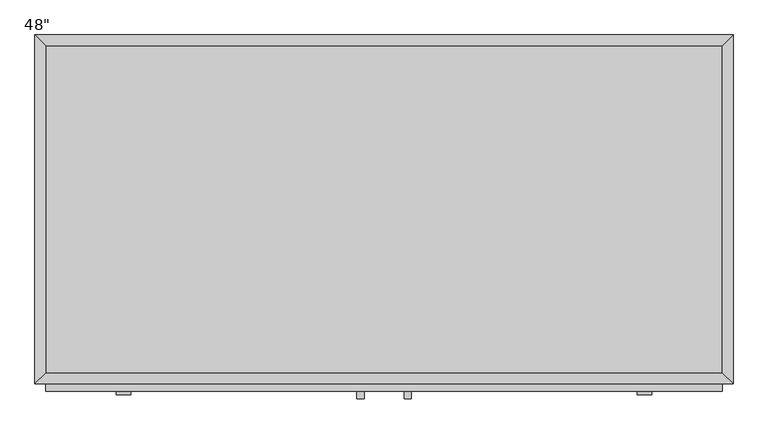
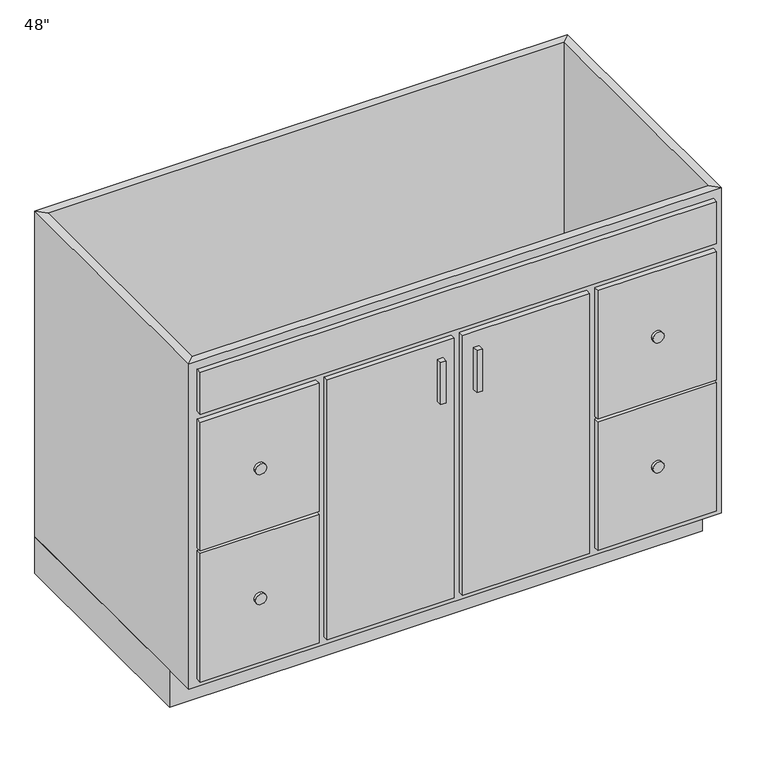
"""IFC4 building model written with IfcOpenShell, lengths in millimetres: furniture geometry."""

from ifc_helpers import new_model, si_unit, point, frame, frame_2d, origin, origin_with_axes, place, context, project, spatial, polyline, circle_curve, trimmed, segment, composite_curve, outline, extrude, faceted_brep, source, transform, mapped, element, save


def furniture_3428e43d(model_context):
    return source(origin(), model_context, "Body", "SolidModel", [
        extrude(outline(polyline([(700.44496, 0.0), (700.44496, -533.4), (-518.75504, -533.4), (-518.75504, 0.0), (700.44496, 0.0)])), origin_with_axes(), (0.0, 0.0, 1.0), 88.9),
        faceted_brep([(681.39496, -590.55, 876.3), (681.39496, -590.55, 88.9), (-499.70504, -590.55, 88.9), (-499.70504, -590.55, 876.3), (700.44496, -609.6, 876.3), (-518.75504, -609.6, 876.3), (700.44496, -609.6, 88.9), (-518.75504, -609.6, 88.9), (-499.70504, -19.05, 88.9), (-499.70504, -19.05, 876.3), (-518.75504, 0.0, 876.3), (-518.75504, 0.0, 88.9), (681.39496, -19.05, 88.9), (681.39496, -19.05, 876.3), (700.44496, 0.0, 876.3), (700.44496, 0.0, 88.9)], [[[0, 1, 2, 3]], [[4, 0, 3, 5]], [[6, 4, 5, 7]], [[1, 6, 7, 2]], [[3, 2, 8, 9]], [[5, 3, 9, 10]], [[7, 5, 10, 11]], [[2, 7, 11, 8]], [[9, 8, 12, 13]], [[10, 9, 13, 14]], [[11, 10, 14, 15]], [[8, 11, 15, 12]], [[13, 12, 1, 0]], [[14, 13, 0, 4]], [[15, 14, 4, 6]], [[12, 15, 6, 1]]]),
        extrude(outline(polyline([(681.39496, -19.05), (681.39496, -590.55), (-499.70504, -590.55), (-499.70504, -19.05), (681.39496, -19.05)])), frame((0.0, 0.0, 88.9), z_axis=(0.0, 0.0, 1.0), x_axis=(1.0, 0.0, 0.0)), (0.0, 0.0, 1.0), 19.05),
        extrude(outline(composite_curve([segment(trimmed(circle_curve(frame_2d((265.1125, 545.66371)), 12.7), [point((265.1125, 532.96371))], [point((265.1125, 558.36371))], False, "CARTESIAN"), True, "CONTINUOUS"), segment(trimmed(circle_curve(frame_2d((265.1125, 545.66371)), 12.7), [point((265.1125, 558.36371))], [point((265.1125, 532.96371))], False, "CARTESIAN"), True, "CONTINUOUS")], self_intersect=False)), frame((0.0, -628.65, 0.0), z_axis=(0.0, 1.0, 0.0), x_axis=(0.0, 0.0, 1.0)), (0.0, 0.0, 1.0), 6.35),
        extrude(outline(composite_curve([segment(trimmed(circle_curve(frame_2d((579.4375, 545.66371)), 12.7), [point((579.4375, 532.96371))], [point((579.4375, 558.36371))], False, "CARTESIAN"), True, "CONTINUOUS"), segment(trimmed(circle_curve(frame_2d((579.4375, 545.66371)), 12.7), [point((579.4375, 558.36371))], [point((579.4375, 532.96371))], False, "CARTESIAN"), True, "CONTINUOUS")], self_intersect=False)), frame((0.0, -628.65, 0.0), z_axis=(0.0, 1.0, 0.0), x_axis=(0.0, 0.0, 1.0)), (0.0, 0.0, 1.0), 6.35),
        extrude(outline(composite_curve([segment(trimmed(circle_curve(frame_2d((579.4375, -363.97379)), 12.7), [point((579.4375, -376.67379))], [point((579.4375, -351.27379))], False, "CARTESIAN"), True, "CONTINUOUS"), segment(trimmed(circle_curve(frame_2d((579.4375, -363.97379)), 12.7), [point((579.4375, -351.27379))], [point((579.4375, -376.67379))], False, "CARTESIAN"), True, "CONTINUOUS")], self_intersect=False)), frame((0.0, -628.65, 0.0), z_axis=(0.0, 1.0, 0.0), x_axis=(0.0, 0.0, 1.0)), (0.0, 0.0, 1.0), 6.35),
        extrude(outline(composite_curve([segment(trimmed(circle_curve(frame_2d((265.1125, -363.97379)), 12.7), [point((265.1125, -376.67379))], [point((265.1125, -351.27379))], False, "CARTESIAN"), True, "CONTINUOUS"), segment(trimmed(circle_curve(frame_2d((265.1125, -363.97379)), 12.7), [point((265.1125, -351.27379))], [point((265.1125, -376.67379))], False, "CARTESIAN"), True, "CONTINUOUS")], self_intersect=False)), frame((0.0, -628.65, 0.0), z_axis=(0.0, 1.0, 0.0), x_axis=(0.0, 0.0, 1.0)), (0.0, 0.0, 1.0), 6.35),
        extrude(outline(polyline([(55.91996, -635.0), (43.21996, -635.0), (43.21996, -622.3), (55.91996, -622.3), (55.91996, -635.0)])), frame((0.0, 0.0, 596.9), z_axis=(0.0, 0.0, 1.0), x_axis=(1.0, 0.0, 0.0)), (0.0, 0.0, 1.0), 101.6),
        extrude(outline(polyline([(138.46996, -635.0), (125.76996, -635.0), (125.76996, -622.3), (138.46996, -622.3), (138.46996, -635.0)])), frame((0.0, 0.0, 596.9), z_axis=(0.0, 0.0, 1.0), x_axis=(1.0, 0.0, 0.0)), (0.0, 0.0, 1.0), 101.6),
        extrude(outline(polyline([(681.39496, -622.3), (-499.70504, -622.3), (-499.70504, -609.6), (681.39496, -609.6), (681.39496, -622.3)])), frame((0.0, 0.0, 755.65), z_axis=(0.0, 0.0, 1.0), x_axis=(1.0, 0.0, 0.0)), (0.0, 0.0, 1.0), 101.6),
        extrude(outline(polyline([(681.39496, -622.3), (409.93246, -622.3), (409.93246, -609.6), (681.39496, -609.6), (681.39496, -622.3)])), frame((0.0, 0.0, 425.45), z_axis=(0.0, 0.0, 1.0), x_axis=(1.0, 0.0, 0.0)), (0.0, 0.0, 1.0), 311.15),
        extrude(outline(polyline([(681.39496, -622.3), (409.93246, -622.3), (409.93246, -609.6), (681.39496, -609.6), (681.39496, -622.3)])), frame((0.0, 0.0, 107.95), z_axis=(0.0, 0.0, 1.0), x_axis=(1.0, 0.0, 0.0)), (0.0, 0.0, 1.0), 311.15),
        extrude(outline(polyline([(-228.24254, -622.3), (-499.70504, -622.3), (-499.70504, -609.6), (-228.24254, -609.6), (-228.24254, -622.3)])), frame((0.0, 0.0, 425.45), z_axis=(0.0, 0.0, 1.0), x_axis=(1.0, 0.0, 0.0)), (0.0, 0.0, 1.0), 311.15),
        extrude(outline(polyline([(-228.24254, -622.3), (-499.70504, -622.3), (-499.70504, -609.6), (-228.24254, -609.6), (-228.24254, -622.3)])), frame((0.0, 0.0, 107.95), z_axis=(0.0, 0.0, 1.0), x_axis=(1.0, 0.0, 0.0)), (0.0, 0.0, 1.0), 311.15),
        extrude(outline(polyline([(81.31996, -622.3), (-209.19254, -622.3), (-209.19254, -609.6), (81.31996, -609.6), (81.31996, -622.3)])), frame((0.0, 0.0, 107.95), z_axis=(0.0, 0.0, 1.0), x_axis=(1.0, 0.0, 0.0)), (0.0, 0.0, 1.0), 628.65),
        extrude(outline(polyline([(390.88246, -622.3), (100.36996, -622.3), (100.36996, -609.6), (390.88246, -609.6), (390.88246, -622.3)])), frame((0.0, 0.0, 107.95), z_axis=(0.0, 0.0, 1.0), x_axis=(1.0, 0.0, 0.0)), (0.0, 0.0, 1.0), 628.65),
    ])


if __name__ == "__main__":
    model = new_model("IFC4")
    model_context = context("Model", 3, world=origin())
    ifc_project = project(units=[si_unit("LENGTHUNIT", "METRE", prefix="MILLI")], contexts=[model_context])
    site = spatial("IfcSite", under=ifc_project)
    building = spatial("IfcBuilding", under=site)
    placement = place(None, origin())
    furniture_shape = furniture_3428e43d(model_context)
    element("IfcFurniture", 1, ObjectType="48\"", at=placement, inside=building, context=model_context, shape_type="MappedRepresentation", body=[
        mapped(furniture_shape, transform((0.0, 0.0, 0.0), x_axis=(1.0, 0.0, 0.0), y_axis=(0.0, 1.0, 0.0), z_axis=(0.0, 0.0, 1.0))),
    ])
    save(model, "model.ifc")

# Revit data of these elements
# Type "48\""
#   Assembly Code = "C1030410"
#   Depth = 2' - 0"
#   Height = 2' - 10 1/2"
#   Toe Depth = 0' - 3"
#   Toe Height = 0' - 3 1/2"
#   Width = 4' - 0"
#   Cabinet Material = none
#   Door/Drawer Material = none
#   Handle Material = Cabinets - Handles
#   Default Elevation = 0
# Element 1 (IfcFurniture, "48\"")
#   Materials on its faces: "Cabinets", "Cabinets - Handles"
# Materials
#   "Cabinets - Handles": class "Metal", colour RGB 57 57 57, transparency 0
#   "Cabinets": colour RGB 249 249 249, transparency 0
